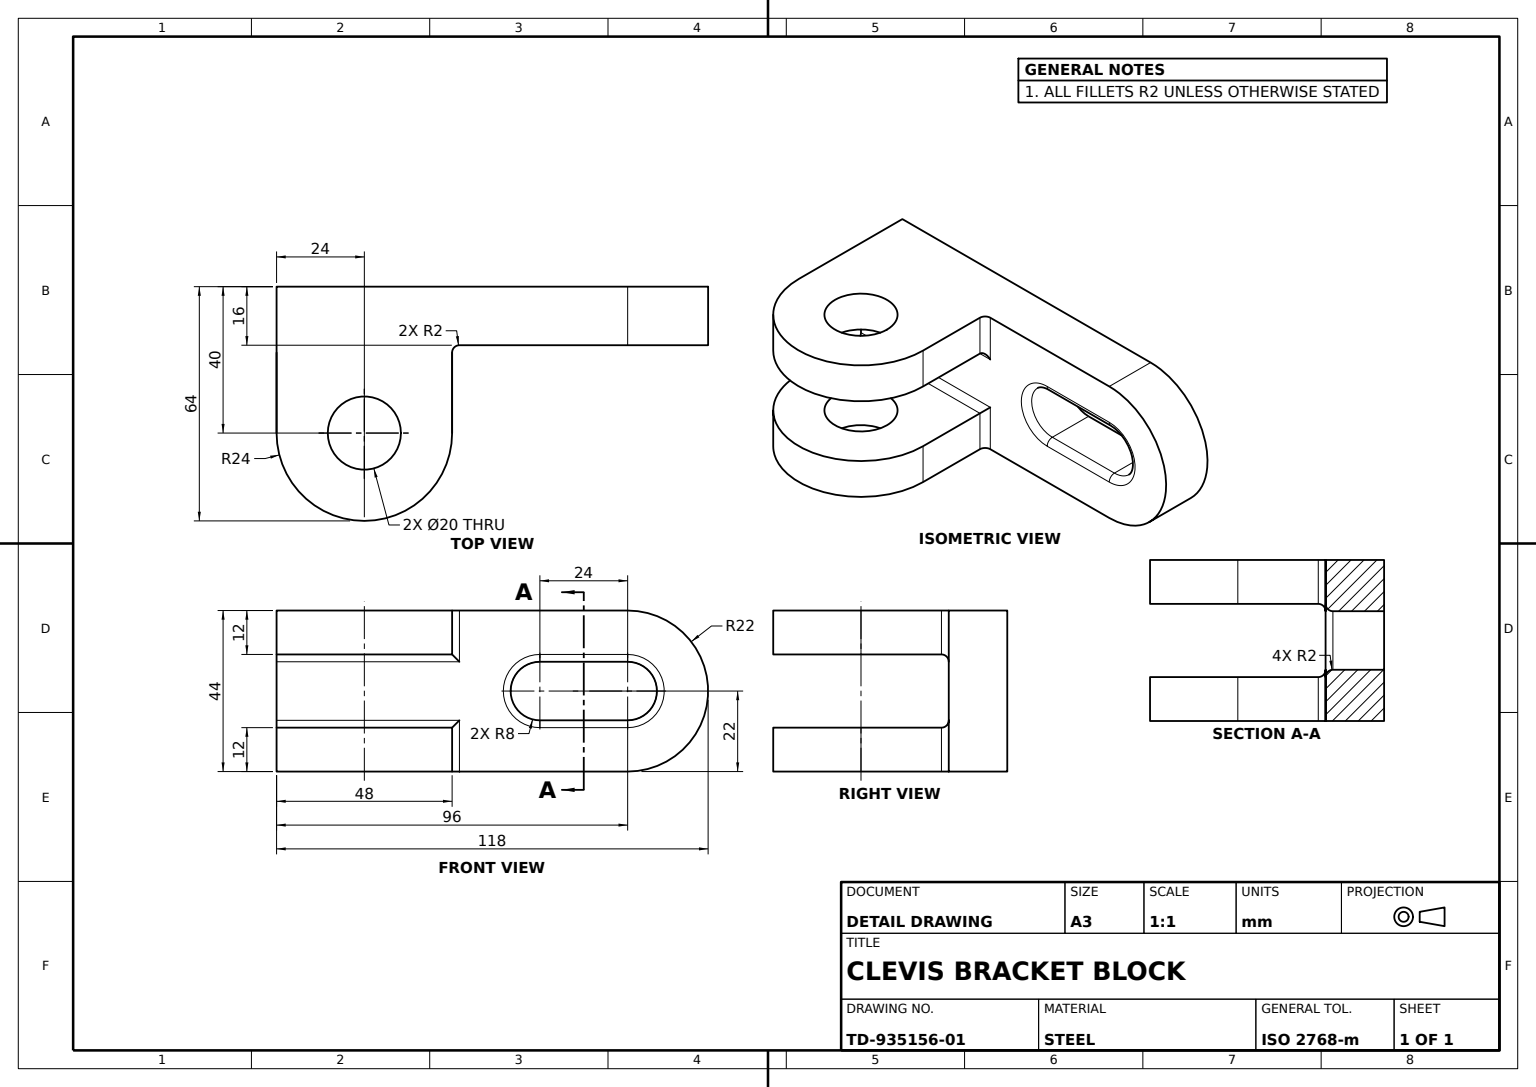
SolidWorks part; units mm, degrees
material "Plain Carbon Steel"
ref_plane "Front Plane" through (0, 0, 0) normal (0, 0, 1) x (1, 0, 0)
ref_plane "Top Plane" through (0, 0, 0) normal (0, 1, 0) x (1, 0, 0)
ref_plane "Right Plane" through (0, 0, 0) normal (1, 0, 0) x (0, 0, -1)
sketch "Base Block Profile" plane through (0, 0, 0) normal (1, 0, 0) x (0, 0, -1)
  line L0 (0, 0) -> (0, 44)
  line L1 (0, 44) -> (96, 44)
  line L2 (96, 0) -> (0, 0)
  arc A0 (96, 44) -> (96, 0) centre (96, 22) cw
  dimension "D1" = 44
  dimension "D2" = 96
  dimension "D3" = 96
extrude "Base Block" add sketch "Base Block Profile" along normal blind 16
sketch "Window Profile" plane through (16, 0, 0) normal (1, 0, 0) x (0, 0, -1)
  line L1 (72, 30) -> (96, 30)
  line L2 (96, 14) -> (72, 14)
  arc A0 (96, 14) -> (96, 30) centre (96, 22) ccw
  arc A1 (72, 30) -> (72, 14) centre (72, 22) ccw
  dimension "D1" = 16
  dimension "D2" = 16
  dimension "D3" = 24
  dimension "D4" = 24
  dimension "D5" = 24
extrude "Base Window Cut" cut sketch "Window Profile" against normal blind 16
sketch "First Lug Profile" plane through (0, 0, 0) normal (0, -1, 0) x (1, 0, 0)
  line L0 (0, 0) -> (40, 0)
  line L1 (40, -48) -> (0, -48)
  line L2 (0, 0) -> (0, -96) construction
  line L3 (0, -48) -> (0, 0)
  arc A0 (40, 0) -> (40, -48) centre (40, -24) cw
  dimension "D1" = 48
  dimension "D2" = 40
extrude "First Lug" add sketch "First Lug Profile" against normal blind 12
sketch "Second Lug Profile" plane through (0, 44, 0) normal (0, 1, 0) x (1, 0, 0)
  line L0 (0, 0) -> (40, 0)
  line L1 (40, 48) -> (0, 48)
  line L2 (0, 96) -> (0, 0) construction
  line L3 (0, 48) -> (0, 0)
  arc A0 (40, 0) -> (40, 48) centre (40, 24) ccw
  arc A1 (40, 0) -> (40, 48) centre (40, 24) ccw construction
extrude "Second Lug" add sketch "Second Lug Profile" against normal blind 12
sketch "Second Lug Hole Profile Ø20" plane through (0, 44, 0) normal (0, 1, 0) x (1, 0, 0)
  circle A0 centre (40, 24) radius 10
  dimension "D1" = 20
extrude "Second Lug Pin Hole Ø20" cut sketch "Second Lug Hole Profile Ø20" against normal blind 12
sketch "First Lug Hole Profile Ø20" plane through (0, 0, 0) normal (0, -1, 0) x (1, 0, 0)
  circle A0 centre (40, -24) radius 10
  dimension "D1" = 20
extrude "First Lug Pin Hole Ø20" cut sketch "First Lug Hole Profile Ø20" against normal blind 12
fillet "First Lug Fillets R2" radius 2 1 edges at (16, 6, -48)
fillet "Lug Junction Fillets R2" radius 2 3 edges at (16, 12, -25) (16, 32, -24) (16, 38, -48)
fillet "Window Edge Fillets R2" radius 2 4 edges at (16, 22, -104) (16, 14, -84) (16, 22, -64) (16, 30, -84)
